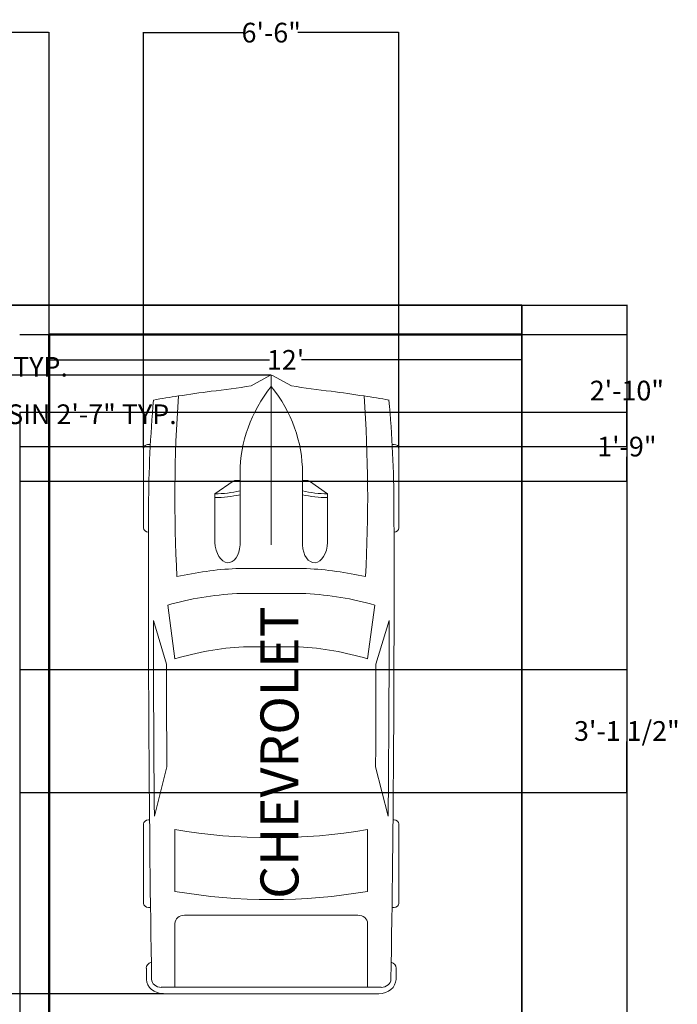
# Model space of a CAD drawing. Units: inches. Extents: x -56 to 545, y -536 to 185.
# Tile 7 of 7: x 345 to 545, y -120 to 180. Entities that reach past the tile are written whole.
import ezdxf

# ---------------------------------------------------------------- set-up
doc = ezdxf.new("R2010")
doc.units = ezdxf.units.IN
doc.header["$MEASUREMENT"] = 0
for name, color, linetype, lineweight in [('A-ANNO-DIMS', 2, 'Continuous', 18), ('A-ANNO-TEXT', 2, 'Continuous', 18), ('A-WALL', 7, 'Continuous', 50), ('C-PRKG-VEHI', 8, 'Continuous', 13), ('C-PROP', 7, 'Continuous', 35)]:
    doc.layers.add(name, color=color, linetype=linetype, lineweight=lineweight)
doc.styles.get("Standard").update_dxf_attribs({"font": 'arial.ttf'})
doc.dimstyles.get("Standard").update_dxf_attribs({"dimtxt": 6, "dimasz": 0.18, "dimexe": 0.18, "dimexo": 0.0625, "dimgap": 0.09, "dimtad": 0, "dimtih": 1, "dimtoh": 1, "dimdec": 0, "dimzin": 0, "dimdsep": 46, "dimlunit": 3, "dimtxsty": 'Standard', "dimcen": 0.09, "dimclrd": 3, "dimclre": 3, "dimclrt": 3, "dimadec": 0, "dimazin": 0, "dimtfac": 1, "dimtdec": 0, "dimtofl": 0, "dimtmove": 0, "dimatfit": 3, "dimfxl": 1, "dimtolj": 1, "dimtzin": 0, "dimarcsym": 0})

# ---------------------------------------------------------------- blocks, each defined once
blk = doc.blocks.new('*U10')
for p, q in [((21.1, 37.41), (21.1, 36.83)), ((46.55, 38.89), (22.35, 38.89)), ((47.8, 37.39), (47.8, 37.41)), ((135.45, 37.07), (135.45, 37.41)), ((136.7, 38.89), (160.9, 38.89)), ((162.15, 37.41), (162.15, 36.77)), ((87.99, 31.87), (74.76, 35.92)), ((134.31, 35.6), (119.29, 31.78)), ((186.47, -33.5), (186.47, 33.5)), ((70.03, 31.54), (86.41, 29.35)), ((188.4, -32.76), (188.4, 32.76)), ((138.42, 29.35), (157.25, 29.35)), ((186.47, 29.35), (167.01, 29.35)), ((164.52, 26.39), (164.52, -26.39)), ((32.27, 11.63), (36.13, 17.17)), ((36.13, 17.17), (50.94, 17.17)), ((29.77, 9.51), (51.68, 9.51)), ((32.12, 9.51), (32.12, 11.15)), ((58.92, -10.77), (58.92, 10.77)), ((66.55, -10.53), (66.55, 10.53)), ((186.47, -10.53), (186.47, 10.53)), ((3.27, 6.13), (0.1, 0.41)), ((82.74, 8.5), (82.74, -8.5)), ((0, 0), (51.68, 0)), ((0.1, -0.41), (3.27, -6.13)), ((29.77, -9.51), (51.68, -9.51)), ((32.12, -9.51), (32.12, -11.15)), ((32.27, -11.63), (36.13, -17.17)), ((36.13, -17.17), (50.94, -17.17)), ((86.41, -29.35), (70.03, -31.54)), ((157.25, -29.35), (138.42, -29.35)), ((167.01, -29.35), (186.47, -29.35)), ((87.99, -31.87), (74.76, -35.92)), ((134.31, -35.6), (119.29, -31.78)), ((21.1, -37.41), (21.1, -36.83)), ((46.55, -38.89), (22.35, -38.89)), ((47.8, -37.39), (47.8, -37.41)), ((135.45, -37.07), (135.45, -37.41)), ((136.7, -38.89), (160.9, -38.89)), ((162.15, -37.41), (162.15, -36.77))]:
    blk.add_line(p, q)
for centre, major_axis, ratio, start_param, end_param in [((41.19, -490.86), (0, 528.23), 0.842304, 0.00281, 0.075598), ((22.35, 37.41), (0, -1.48), 0.842304, 3.141593, 4.712389), ((64.48, -10555.62), (0, 10593.03), 0.842304, -0.013397, 0.002797), ((46.55, 37.41), (0, 1.48), 0.842304, -1.570796, 0), ((136.7, 37.41), (0, -1.48), 0.842304, 3.141593, 4.712389), ((160.9, 37.41), (0, 1.48), 0.842304, -1.570796, 0), ((180.63, 35.84), (0, 2.22), 0.842304, -0.013017, 1.249894), ((64.48, -10556.36), (0, 10595.31), 0.842304, -0.013397, -0.013017), ((183.98, 33.5), (0, -2.96), 0.842304, 1.570796, 3.128196), ((183.98, 32.76), (0, -5.25), 0.842304, 1.570796, 3.128196), ((266.03, -27.52), (0, 313.31), 0.842304, 1.367076, 1.39176), ((64.48, -10555.62), (0, -10591.55), 0.842304, 3.133765, 3.140441), ((135.29, 5.39), (0, 81.77), 0.842304, 1.245306, 1.50788), ((95.79, -3666.35), (0, -3698.24), 0.842304, 3.134049, 3.144098), ((259.18, -27.52), (0, -305.3), 0.842304, 4.528606, 4.561838), ((37.47, -593.96), (0, -623.33), 0.842304, 3.096046, 3.200911), ((134.4, 5.39), (0, -89.78), 0.842304, 4.449482, 4.652344), ((149.6, 2.8), (0, -79.58), 0.842304, 4.372215, 4.640744), ((17.08, 0), (0, 147.02), 0.842304, 4.511394, 4.913384), ((35.91, 0), (0, 147.02), 0.842304, 4.511394, 4.913384), ((167.01, 26.39), (0, 2.96), 0.842304, 0, 1.570796), ((-204.49, 52.4), (0, -250.96), 0.842304, 1.385369, 1.434372), ((13.04, 17.01), (0, 27.42), 0.842304, 4.435146, 4.718221), ((14.2, 17.01), (0, 27.42), 0.842304, 4.435146, 4.718221), ((50.79, 13.34), (6.34, -0.36), 0.603834, -1.395552, 1.581315), ((29.77, -46.66), (0, 56.17), 0.842304, 0, 0.590319), ((32.75, 11.15), (0, 0.74), 0.842304, 0.879714, 1.570796), ((0.62, 0), (0, -0.74), 0.842304, 4.131459, 5.293319), ((29.77, 46.66), (0, 56.17), 0.842304, 2.551274, 3.141593), ((-204.49, -52.4), (0, 250.96), 0.842304, -1.434372, -1.385369), ((149.6, -2.8), (0, -79.58), 0.842304, -1.499151, -1.230623), ((32.75, -11.15), (0, -0.74), 0.842304, 4.712389, 5.403472), ((13.04, -17.01), (0, -27.42), 0.842304, 1.564964, 1.848039), ((14.2, -17.01), (0, -27.42), 0.842304, 1.564964, 1.848039), ((134.4, -5.39), (0, -89.78), 0.842304, -1.510751, -1.307889), ((135.29, -5.39), (0, -81.77), 0.842304, -1.50788, -1.245306), ((259.18, 27.52), (0, 305.3), 0.842304, 1.721348, 1.754579), ((167.01, -26.39), (0, -2.96), 0.842304, 4.712389, 6.283185), ((266.03, 27.52), (0, 313.31), 0.842304, 1.749832, 1.774517), ((37.47, 593.96), (0, -623.33), 0.842304, -0.059319, 0.045547), ((95.79, 3666.35), (0, -3698.24), 0.842304, -0.002505, 0.007544), ((183.98, -32.76), (0, -5.25), 0.842304, 0.013397, 1.570796), ((41.19, 490.86), (0, -528.23), 0.842304, -0.075598, -0.00281), ((64.48, 10555.62), (0, -10591.55), 0.842304, 0.001152, 0.007828), ((183.98, -33.5), (0, 2.96), 0.842304, 3.15499, 4.712389), ((22.35, -37.41), (0, 1.48), 0.842304, 1.570796, 3.141593), ((64.48, 10555.62), (0, 10593.03), 0.842304, 3.138796, 3.15499), ((46.55, -37.41), (0, -1.48), 0.842304, 0, 1.570796), ((136.7, -37.41), (0, -1.48), 0.842304, -1.570796, 0), ((160.9, -37.41), (0, 1.48), 0.842304, 3.141593, 4.712389), ((180.63, -35.84), (0, -2.22), 0.842304, -1.249894, 0.013017), ((64.48, 10556.36), (0, 10595.31), 0.842304, 3.15461, 3.15499)]:
    blk.add_ellipse(centre, major_axis=major_axis, ratio=ratio, start_param=start_param, end_param=end_param)
at = {"extrusion": (0, 0, -1)}
blk.add_ellipse((50.79, -13.34), major_axis=(6.34, 0.36), ratio=0.603834, start_param=-1.395552, end_param=1.581315, dxfattribs=at)
blk = doc.blocks.new('*D35')
at = {"layer": 'A-ANNO-DIMS', "color": 0, "lineweight": -2, "transparency": 16777216}
for p, q in [((354.03, 76.51), (354.03, 76.63)), ((354.21, 76.45), (421.14, 76.45)), ((497.85, 76.45), (430.93, 76.45)), ((498.03, 76.51), (498.03, 76.63))]:
    blk.add_line(p, q, dxfattribs=at)
at = {"layer": 'A-ANNO-DIMS', "color": 0, "transparency": 16777216}
for points in [[(354.21, 76.48), (354.21, 76.42), (354.03, 76.45)], [(497.85, 76.48), (497.85, 76.42), (498.03, 76.45)]]:
    blk.add_solid(points, dxfattribs=at)
at = {"layer": 'Defpoints', "color": 0, "transparency": 16777216}
for p in [(354.03, 76.45), (498.03, 76.45), (498.03, 76.45)]:
    blk.add_point(p, dxfattribs=at)
at = {"layer": 'A-ANNO-DIMS', "color": 0, "transparency": 16777216, "insert": (426.03, 76.45), "char_height": 6, "attachment_point": 5}
blk.add_mtext("\\A1;12'", dxfattribs=at)
blk = doc.blocks.new('*D39')
at = {"layer": 'A-ANNO-DIMS', "color": 3, "lineweight": -2, "transparency": 16777216}
for p, q in [((298.63, 64.49), (298.63, 59.71)), ((329.69, 64.49), (329.69, 59.71)), ((298.81, 59.89), (329.51, 59.89)), ((329.69, 59.89), (329.87, 59.89))]:
    blk.add_line(p, q, dxfattribs=at)
at = {"layer": 'A-ANNO-DIMS', "color": 3, "transparency": 16777216}
for points in [[(298.81, 59.92), (298.81, 59.86), (298.63, 59.89)], [(329.51, 59.92), (329.51, 59.86), (329.69, 59.89)]]:
    blk.add_solid(points, dxfattribs=at)
at = {"layer": 'Defpoints', "color": 0, "transparency": 16777216}
for p in [(298.63, 64.55), (329.69, 64.55), (329.69, 59.89)]:
    blk.add_point(p, dxfattribs=at)
at = {"layer": 'A-ANNO-DIMS', "color": 3, "transparency": 16777216, "insert": (361.86, 59.89), "char_height": 6, "attachment_point": 5}
blk.add_mtext('\\A1;BASIN 2\'-7" TYP.', dxfattribs=at)
blk = doc.blocks.new('*D40')
at = {"layer": 'A-ANNO-DIMS', "color": 3, "lineweight": -2, "transparency": 16777216}
for p, q in [((329.75, 84.16), (334.53, 84.16)), ((334.35, 83.98), (334.35, 77.55)), ((334.35, 64.73), (334.35, 71.16)), ((329.75, 64.55), (334.53, 64.55))]:
    blk.add_line(p, q, dxfattribs=at)
at = {"layer": 'A-ANNO-DIMS', "color": 3, "transparency": 16777216}
for points in [[(334.32, 83.98), (334.38, 83.98), (334.35, 84.16)], [(334.32, 64.73), (334.38, 64.73), (334.35, 64.55)]]:
    blk.add_solid(points, dxfattribs=at)
at = {"layer": 'Defpoints', "color": 0, "transparency": 16777216}
for p in [(329.69, 84.16), (334.35, 84.16), (329.69, 64.55)]:
    blk.add_point(p, dxfattribs=at)
at = {"layer": 'A-ANNO-DIMS', "color": 3, "transparency": 16777216, "insert": (334.35, 74.35), "char_height": 6, "attachment_point": 5}
blk.add_mtext('\\A1;1\'-7 1/2" TYP.', dxfattribs=at)
blk = doc.blocks.new('*D70')
at = {"layer": 'A-ANNO-DIMS', "color": 3, "lineweight": -2, "transparency": 16777216}
for p, q in [((421.61, 71.8), (-38.11, 71.8)), ((-37.93, 71.62), (-37.93, -19.2)), ((-37.93, -116.42), (-37.93, -25.59)), ((388.85, -116.6), (-38.11, -116.6))]:
    blk.add_line(p, q, dxfattribs=at)
at = {"layer": 'A-ANNO-DIMS', "color": 3, "transparency": 16777216}
for points in [[(-37.96, 71.62), (-37.9, 71.62), (-37.93, 71.8)], [(-37.96, -116.42), (-37.9, -116.42), (-37.93, -116.6)]]:
    blk.add_solid(points, dxfattribs=at)
at = {"layer": 'Defpoints', "color": 0, "transparency": 16777216}
for p in [(421.67, 71.8), (-37.93, -116.6), (388.91, -116.6)]:
    blk.add_point(p, dxfattribs=at)
at = {"layer": 'A-ANNO-DIMS', "color": 3, "transparency": 16777216, "insert": (-37.93, -22.4), "char_height": 6, "attachment_point": 5}
blk.add_mtext('\\A1;15\'-8 1/2"', dxfattribs=at)
blk = doc.blocks.new('*D71')
at = {"layer": 'A-ANNO-DIMS', "color": 3, "lineweight": -2, "transparency": 16777216}
for p, q in [((382.78, 49.51), (382.78, 176.3)), ((382.96, 176.12), (413.59, 176.12)), ((460.38, 176.12), (429.75, 176.12)), ((460.56, 49.51), (460.56, 176.3))]:
    blk.add_line(p, q, dxfattribs=at)
at = {"layer": 'A-ANNO-DIMS', "color": 3, "transparency": 16777216}
for points in [[(382.96, 176.15), (382.96, 176.09), (382.78, 176.12)], [(460.38, 176.15), (460.38, 176.09), (460.56, 176.12)]]:
    blk.add_solid(points, dxfattribs=at)
at = {"layer": 'Defpoints', "color": 0, "transparency": 16777216}
for p in [(460.56, 176.12), (382.78, 49.45), (460.56, 49.45)]:
    blk.add_point(p, dxfattribs=at)
at = {"layer": 'A-ANNO-DIMS', "color": 3, "transparency": 16777216, "insert": (421.67, 176.12), "char_height": 6, "attachment_point": 5}
blk.add_mtext('\\A1;6\'-6"', dxfattribs=at)
blk = doc.blocks.new('*D80')
at = {"layer": 'A-ANNO-DIMS', "color": 3, "lineweight": -2, "transparency": 16777216}
for p, q in [((345.1, 84.16), (530.18, 84.16)), ((530, 83.98), (530, 70.25)), ((530, 50.21), (530, 63.94)), ((345.1, 50.03), (530.18, 50.03))]:
    blk.add_line(p, q, dxfattribs=at)
at = {"layer": 'A-ANNO-DIMS', "color": 3, "transparency": 16777216}
for points in [[(529.97, 83.98), (530.03, 83.98), (530, 84.16)], [(529.97, 50.21), (530.03, 50.21), (530, 50.03)]]:
    blk.add_solid(points, dxfattribs=at)
at = {"layer": 'Defpoints', "color": 0, "transparency": 16777216}
for p in [(345.03, 84.16), (530, 84.16), (345.03, 50.03)]:
    blk.add_point(p, dxfattribs=at)
at = {"layer": 'A-ANNO-DIMS', "color": 3, "transparency": 16777216, "insert": (530, 67.09), "char_height": 6, "attachment_point": 5}
blk.add_mtext('\\A1;2\'-10"', dxfattribs=at)
blk = doc.blocks.new('*D81')
at = {"layer": 'A-ANNO-DIMS', "color": 3, "lineweight": -2, "transparency": 16777216}
for p, q in [((345.03, 60.47), (345.03, -526.99)), ((312.03, 49.97), (312.03, -526.99)), ((312.21, -526.81), (320.42, -526.81)), ((344.85, -526.81), (336.65, -526.81))]:
    blk.add_line(p, q, dxfattribs=at)
at = {"layer": 'A-ANNO-DIMS', "color": 3, "transparency": 16777216}
for points in [[(312.21, -526.78), (312.21, -526.84), (312.03, -526.81)], [(344.85, -526.78), (344.85, -526.84), (345.03, -526.81)]]:
    blk.add_solid(points, dxfattribs=at)
at = {"layer": 'Defpoints', "color": 0, "transparency": 16777216}
for p in [(345.03, 60.53), (312.03, 50.03), (312.03, -526.81)]:
    blk.add_point(p, dxfattribs=at)
at = {"layer": 'A-ANNO-DIMS', "color": 3, "transparency": 16777216, "insert": (328.53, -526.81), "char_height": 6, "attachment_point": 5}
blk.add_mtext('\\A1;2\'-9"', dxfattribs=at)
blk = doc.blocks.new('*D82')
at = {"layer": 'A-ANNO-DIMS', "color": 3, "lineweight": -2, "transparency": 16777216}
for p, q in [((345.1, 60.53), (530.18, 60.53)), ((530, 60.35), (530, 53.18)), ((530, 39.71), (530, 46.88)), ((345.1, 39.53), (530.18, 39.53))]:
    blk.add_line(p, q, dxfattribs=at)
at = {"layer": 'A-ANNO-DIMS', "color": 3, "transparency": 16777216}
for points in [[(529.97, 60.35), (530.03, 60.35), (530, 60.53)], [(529.97, 39.71), (530.03, 39.71), (530, 39.53)]]:
    blk.add_solid(points, dxfattribs=at)
at = {"layer": 'Defpoints', "color": 0, "transparency": 16777216}
for p in [(345.03, 60.53), (345.03, 39.53), (530, 39.53)]:
    blk.add_point(p, dxfattribs=at)
at = {"layer": 'A-ANNO-DIMS', "color": 3, "transparency": 16777216, "insert": (530, 50.03), "char_height": 6, "attachment_point": 5}
blk.add_mtext('\\A1;1\'-9"', dxfattribs=at)
blk = doc.blocks.new('*D87')
at = {"layer": 'A-ANNO-DIMS', "color": 3, "lineweight": -2, "transparency": 16777216}
for p, q in [((345.1, -17.84), (530.18, -17.84)), ((530, -18.02), (530, -33.4)), ((530, -55.16), (530, -39.78)), ((345.1, -55.34), (530.18, -55.34))]:
    blk.add_line(p, q, dxfattribs=at)
at = {"layer": 'A-ANNO-DIMS', "color": 3, "transparency": 16777216}
for points in [[(529.97, -18.02), (530.03, -18.02), (530, -17.84)], [(529.97, -55.16), (530.03, -55.16), (530, -55.34)]]:
    blk.add_solid(points, dxfattribs=at)
at = {"layer": 'Defpoints', "color": 0, "transparency": 16777216}
for p in [(345.03, -17.84), (345.03, -55.34), (530, -55.34)]:
    blk.add_point(p, dxfattribs=at)
at = {"layer": 'A-ANNO-DIMS', "color": 3, "transparency": 16777216, "insert": (530, -36.59), "char_height": 6, "attachment_point": 5}
blk.add_mtext('\\A1;3\'-1 1/2"', dxfattribs=at)
blk = doc.blocks.new('*D90')
at = {"layer": 'A-ANNO-DIMS', "color": 3, "lineweight": -2, "transparency": 16777216}
for p, q in [((-5.97, 93.22), (-5.97, 176.3)), ((-5.79, 176.12), (163.64, 176.12)), ((353.85, 176.12), (184.43, 176.12)), ((354.03, 84.22), (354.03, 176.3))]:
    blk.add_line(p, q, dxfattribs=at)
at = {"layer": 'A-ANNO-DIMS', "color": 3, "transparency": 16777216}
for points in [[(-5.79, 176.15), (-5.79, 176.09), (-5.97, 176.12)], [(353.85, 176.15), (353.85, 176.09), (354.03, 176.12)]]:
    blk.add_solid(points, dxfattribs=at)
at = {"layer": 'Defpoints', "color": 0, "transparency": 16777216}
for p in [(354.03, 176.12), (-5.97, 93.16), (354.03, 84.16)]:
    blk.add_point(p, dxfattribs=at)
at = {"layer": 'A-ANNO-DIMS', "color": 3, "transparency": 16777216, "insert": (174.03, 176.12), "char_height": 6, "attachment_point": 5}
blk.add_mtext('\\A1;30\'-0"', dxfattribs=at)
blk = doc.blocks.new('*D91')
at = {"layer": 'A-ANNO-DIMS', "color": 3, "lineweight": -2, "transparency": 16777216}
for p, q in [((498.1, 93.16), (530.18, 93.16)), ((530, 92.98), (530, -160.19)), ((530, -419.66), (530, -166.49)), ((354.1, -419.84), (530.18, -419.84))]:
    blk.add_line(p, q, dxfattribs=at)
at = {"layer": 'A-ANNO-DIMS', "color": 3, "transparency": 16777216}
for points in [[(529.97, 92.98), (530.03, 92.98), (530, 93.16)], [(529.97, -419.66), (530.03, -419.66), (530, -419.84)]]:
    blk.add_solid(points, dxfattribs=at)
at = {"layer": 'Defpoints', "color": 0, "transparency": 16777216}
for p in [(498.03, 93.16), (354.03, -419.84), (530, -419.84)]:
    blk.add_point(p, dxfattribs=at)
at = {"layer": 'A-ANNO-DIMS', "color": 3, "transparency": 16777216, "insert": (530, -163.34), "char_height": 6, "attachment_point": 5}
blk.add_mtext('\\A1;42\'-9"', dxfattribs=at)

msp = doc.modelspace()

# ---------------------------------------------------------------- linework, layer by layer
at = {"layer": 'A-WALL'}
for q in [(498.03, 84.16), (354.03, -494.84)]:
    msp.add_line((354.03, 84.16), q, dxfattribs=at)
at = {"layer": 'C-PROP'}
for p, q in [((-5.97, 93.16), (498.03, 93.16)), ((498.03, 93.16), (498.03, -491.84))]:
    msp.add_line(p, q, dxfattribs=at)

# ---------------------------------------------------------------- block references
at = {"layer": 'C-PRKG-VEHI', "rotation": 270}
msp.add_blockref('*U10', (421.67, 71.8), dxfattribs=at)

# ---------------------------------------------------------------- texts
at = {"layer": 'A-ANNO-TEXT', "insert": (418.38, -87.72), "char_height": 11.5844, "attachment_point": 1, "rotation": 90}
msp.add_mtext_dynamic_manual_height_columns('{\\fArial|b1|i0|c0|p34;CHEVROLET}', width=2189.6751, gutter_width=57.92, heights=[0], dxfattribs=at)

# ---------------------------------------------------------------- dimensions: what is measured, and where the dimension line sits
at = {"layer": 'A-ANNO-DIMS'}
for base, p1, p2, override, picture, middle in [((354.03, 176.12), (-5.97, 93.16), (354.03, 84.16), {"dimdec": 1, "dimlfac": 1, "dimrnd": 0, "dimzin": 1, "dimdsep": 46, "dimlunit": 4, "dimfrac": 2}, '*D90', (174.03, 176.12)), ((460.56, 176.12), (382.78, 49.45), (460.56, 49.45), {"dimdec": 1, "dimlfac": 1, "dimrnd": 0, "dimzin": 1, "dimdsep": 46, "dimlunit": 4, "dimfrac": 2}, '*D71', (421.67, 176.12)), ((498.03, 76.45), (354.03, 76.45), (498.03, 76.45), {"dimclrd": 0, "dimclre": 0, "dimclrt": 0}, '*D35', (426.03, 76.45)), ((312.03, -526.81), (345.03, 60.53), (312.03, 50.03), {"dimdec": 1, "dimlfac": 1, "dimrnd": 0, "dimzin": 1, "dimdsep": 46, "dimlunit": 4, "dimfrac": 2}, '*D81', (328.53, -526.81))]:
    dim = msp.add_linear_dim(base=base, p1=p1, p2=p2, dimstyle='Standard', override=override, dxfattribs=at)
    dim.commit()
    dim.dimension.update_dxf_attribs({"geometry": picture, "text_midpoint": middle})
for base, p1, p2, picture, middle in [((530, -419.84), (498.03, 93.16), (354.03, -419.84), '*D91', (530, -163.34)), ((530, 84.16), (345.03, 50.03), (345.03, 84.16), '*D80', (530, 67.09)), ((-37.93, -116.6), (421.67, 71.8), (388.91, -116.6), '*D70', (-37.93, -22.4)), ((530, 39.53), (345.03, 60.53), (345.03, 39.53), '*D82', (530, 50.03)), ((530, -55.34), (345.03, -17.84), (345.03, -55.34), '*D87', (530, -36.59))]:
    dim = msp.add_linear_dim(base=base, p1=p1, p2=p2, angle=90, dimstyle='Standard', override={"dimdec": 1, "dimlfac": 1, "dimrnd": 0, "dimzin": 1, "dimdsep": 46, "dimlunit": 4, "dimfrac": 2}, dxfattribs=at)
    dim.commit()
    dim.dimension.update_dxf_attribs({"geometry": picture, "text_midpoint": middle})
dim = msp.add_linear_dim(base=(334.35, 84.16), p1=(329.69, 64.55), p2=(329.69, 84.16), angle=90, text='<> TYP.', dimstyle='Standard', override={"dimdec": 1, "dimlfac": 1, "dimrnd": 0, "dimzin": 1, "dimdsep": 46, "dimlunit": 4, "dimfrac": 2}, dxfattribs=at)
dim.commit()
dim.dimension.update_dxf_attribs({"geometry": '*D40', "text_midpoint": (334.35, 74.35)})
dim = msp.add_linear_dim(base=(329.69, 59.89), p1=(298.63, 64.55), p2=(329.69, 64.55), text='BASIN <> TYP.', dimstyle='Standard', override={"dimdec": 1, "dimlfac": 1, "dimrnd": 0, "dimzin": 1, "dimdsep": 46, "dimlunit": 4, "dimfrac": 2}, dxfattribs=at)
dim.commit()
dim.dimension.update_dxf_attribs({"geometry": '*D39', "text_midpoint": (361.86, 59.89)})

doc.saveas('drawing.dxf')
